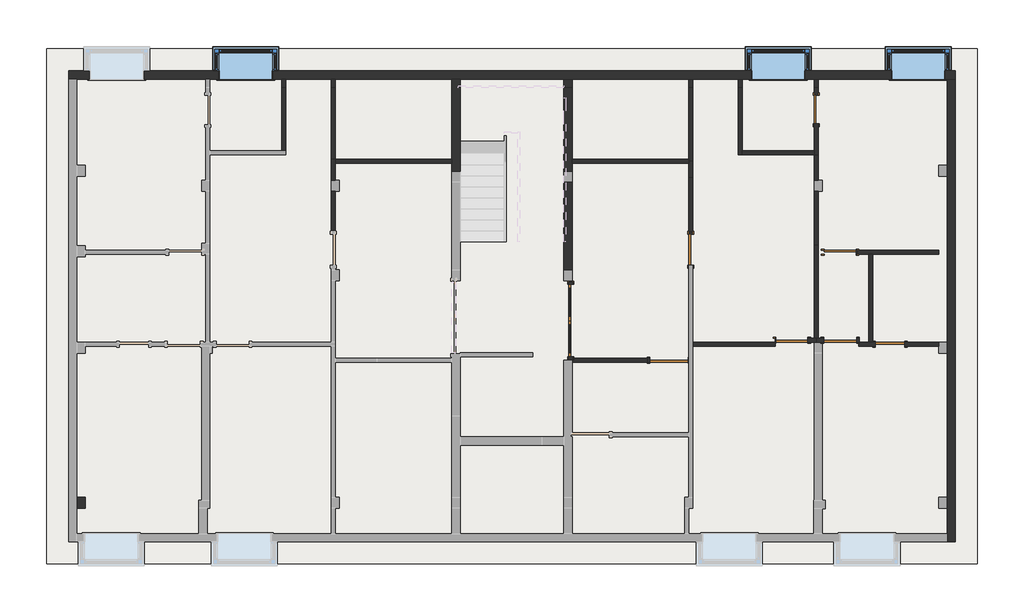
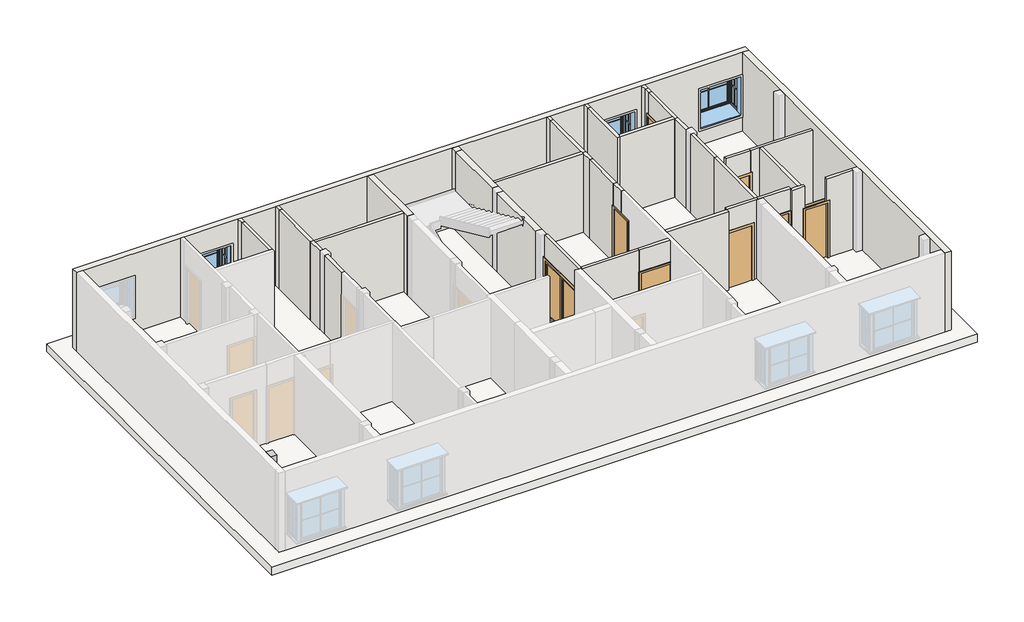
# One storey, part 2 of 3: 39 walls, 8 doors, 3 windows, 1 column, 1 slab.
"""IFC4 building model written with IfcOpenShell, lengths in millimetres."""

from ifc_helpers import new_model, si_unit, frame, origin, place, context, project, spatial, polyline, outline, extrude, faceted_brep, transform, mapped, element, save
from components import door_04ab2522, m_door_single_panel_05506f71, door_85b31ab1, door_1991e9a2, door_a431d384, door_82def9da, m_door_single_panel_3_x7_f8176753, window_19bbd869

model = new_model("IFC4")

# Units and contexts
model_context = context("Model", 3, world=origin())
ifc_project = project(units=[si_unit("LENGTHUNIT", "METRE", prefix="MILLI")], contexts=[model_context])

# Site, building, storey
site = spatial("IfcSite", under=ifc_project)
building = spatial("IfcBuilding", under=site)
storey = spatial("IfcBuildingStorey", under=building, Elevation=19202.4)

# Column
placement = place(None, origin())
element("IfcColumn", 1, ObjectType="Rectangular Column : 1'X 9\"", at=placement, inside=storey, context=model_context, shape_type="SweptSolid", body=[
    extrude(outline(polyline([(-12224.6987957, -3709.2932671), (-12224.6987957, -4014.0932671), (-12453.2987957, -4014.0932671), (-12453.2987957, -3709.2932671), (-12224.6987957, -3709.2932671)])), frame((0.0, 0.0, 19202.4), z_axis=(0.0, 0.0, 1.0), x_axis=(1.0, 0.0, 0.0)), (0.0, 0.0, 1.0), 3048.0),
])

# Doors
door_shape = door_04ab2522(model_context)
element("IfcDoor", 2, ObjectType="M_Door-Double-Glass : 6'7\"X7'", at=placement, inside=storey, context=model_context, shape_type="MappedRepresentation", body=[
    mapped(door_shape, transform((1217.5394962, 1183.3817656, 19202.4), x_axis=(0.0, 1.0, 0.0), y_axis=(-1.0, 0.0, 0.0), z_axis=(0.0, 0.0, 1.0))),
])
m_door_single_panel_shape = m_door_single_panel_05506f71(model_context)
element("IfcDoor", 3, ObjectType="M_Door-Single-Panel", at=placement, inside=storey, context=model_context, shape_type="MappedRepresentation", body=[
    mapped(m_door_single_panel_shape, transform((3933.4813133, 90.9578621, 19202.4), x_axis=(1.0, 0.0, 0.0), y_axis=(0.0, 1.0, 0.0), z_axis=(0.0, 0.0, 1.0))),
])
door_2_shape = door_85b31ab1(model_context)
element("IfcDoor", 4, ObjectType="M_Door-Single-Panel : 2'10\"X7' 2", at=placement, inside=storey, context=model_context, shape_type="MappedRepresentation", body=[
    mapped(door_2_shape, transform((4532.9512082, 3142.9626891, 19202.4), x_axis=(0.0, -1.0, 0.0), y_axis=(1.0, 0.0, 0.0), z_axis=(0.0, 0.0, 1.0))),
])
door_3_shape = door_1991e9a2(model_context)
element("IfcDoor", 5, ObjectType="M_Door-Single-Panel : 2'11\"X7' 3", at=placement, inside=storey, context=model_context, shape_type="MappedRepresentation", body=[
    mapped(door_3_shape, transform((7330.1405552, 640.4567334, 19202.4), x_axis=(1.0, 0.0, 0.0), y_axis=(0.0, 1.0, 0.0), z_axis=(0.0, 0.0, 1.0))),
])
element("IfcDoor", 6, ObjectType="M_Door-Single-Panel : 2'11\"X7' 3", at=placement, inside=storey, context=model_context, shape_type="MappedRepresentation", body=[
    mapped(door_3_shape, transform((8664.274939, 3078.8567332, 19202.4), x_axis=(-1.0, 0.0, 0.0), y_axis=(0.0, -1.0, 0.0), z_axis=(0.0, 0.0, 1.0))),
])
door_4_shape = door_a431d384(model_context)
element("IfcDoor", 7, ObjectType="M_Door-Single-Panel : 2'7\"X7' 2", at=placement, inside=storey, context=model_context, shape_type="MappedRepresentation", body=[
    mapped(door_4_shape, transform((8000.0512079, 7021.3751452, 19202.4), x_axis=(0.0, 1.0, 0.0), y_axis=(-1.0, 0.0, 0.0), z_axis=(0.0, 0.0, 1.0))),
])
door_5_shape = door_82def9da(model_context)
element("IfcDoor", 8, ObjectType="M_Door-Single-Panel : 2'8\"X7'", at=placement, inside=storey, context=model_context, shape_type="MappedRepresentation", body=[
    mapped(door_5_shape, transform((10046.0486694, 526.1567295, 19202.4), x_axis=(-1.0, 0.0, 0.0), y_axis=(0.0, -1.0, 0.0), z_axis=(0.0, 0.0, 1.0))),
])
m_door_single_panel_3_x7_shape = m_door_single_panel_3_x7_f8176753(model_context)
element("IfcDoor", 9, ObjectType="M_Door-Single-Panel : 3'X7'", at=placement, inside=storey, context=model_context, shape_type="MappedRepresentation", body=[
    mapped(m_door_single_panel_3_x7_shape, transform((8666.8012079, 640.4567334, 19202.4), x_axis=(-1.0, 0.0, 0.0), y_axis=(0.0, -1.0, 0.0), z_axis=(0.0, 0.0, 1.0))),
])

# Slab
element("IfcSlab", 10, ObjectType="Generic - 12\"", at=placement, inside=storey, context=model_context, shape_type="SweptSolid", body=[
    extrude(outline(polyline([(12464.1012075, 8698.6067329), (12464.1012075, -5550.7932662), (-13291.4987957, -5550.7932662), (-13291.4987957, 8698.6067329), (12464.1012075, 8698.6067329)])), frame((0.0, 0.0, 18897.6), z_axis=(0.0, 0.0, 1.0), x_axis=(1.0, 0.0, 0.0)), (0.0, 0.0, 1.0), 304.8),
])

# Walls
element("IfcWall", 11, ObjectType="4.5\"", at=placement, inside=storey, context=model_context, shape_type="SweptSolid", body=[
    extrude(outline(polyline([(3132.0737955, 22250.4), (3628.3344162, 22250.4), (3628.3344162, 19202.4), (3574.7626891, 19202.4), (3574.7626891, 21336.0), (3132.0737955, 21336.0), (3132.0737955, 22250.4)])), frame((4475.8012082, 0.0, 0.0), z_axis=(1.0, 0.0, 0.0), x_axis=(0.0, 1.0, 0.0)), (0.0, 0.0, 1.0), 114.3),
])
element("IfcWall", 12, ObjectType="4.5\"", at=placement, inside=storey, context=model_context, shape_type="Brep", body=[
    faceted_brep([(8000.0512079, 583.3067334, 19202.4), (8000.0512079, 583.3067334, 22250.4), (7942.9012047, 583.3067334, 22250.4), (6862.7668241, 583.3067334, 22250.4), (6862.7668241, 583.3067334, 19202.4), (6885.6405552, 583.3067334, 19202.4), (6885.6405552, 583.3067334, 21336.0), (7774.6405552, 583.3067334, 21336.0), (7774.6405552, 583.3067334, 19202.4), (7942.9012047, 583.3067334, 19202.4), (8000.0512079, 697.6067334, 22250.4), (8000.0512079, 697.6067334, 19202.4), (7942.9012079, 697.6067334, 19202.4), (7774.6405552, 697.6067334, 19202.4), (7774.6405552, 697.6067334, 21336.0), (6885.6405552, 697.6067334, 21336.0), (6885.6405552, 697.6067334, 19202.4), (6862.7668241, 697.6067334, 19202.4), (6862.7668241, 697.6067334, 22250.4), (7942.9012079, 697.6067334, 22250.4)], [[[0, 1, 2, 3, 4, 5, 6, 7, 8, 9]], [[10, 11, 12, 13, 14, 15, 16, 17, 18, 19]], [[4, 17, 16, 5]], [[11, 0, 9, 8, 13, 12]], [[1, 0, 11, 10]], [[3, 2, 1, 10, 19, 18]], [[4, 3, 18, 17]], [[7, 14, 13, 8]], [[14, 7, 6, 15]], [[15, 6, 5, 16]]]),
])
element("IfcWall", 13, ObjectType="4.5\"", at=placement, inside=storey, context=model_context, shape_type="Brep", body=[
    faceted_brep([(9187.5012047, 583.3067334, 19202.4), (9187.5012047, 583.3067334, 22250.4), (8171.5012047, 583.3067334, 22250.4), (8000.0512079, 583.3067334, 22250.4), (8000.0512079, 583.3067334, 19202.4), (8171.5012047, 583.3067334, 19202.4), (8209.6012079, 583.3067334, 19202.4), (8209.6012079, 583.3067334, 21336.0), (9124.0012079, 583.3067334, 21336.0), (9124.0012079, 583.3067334, 19202.4), (9187.5012047, 697.6067334, 22250.4), (9187.5012047, 697.6067334, 19202.4), (9124.0012079, 697.6067334, 19202.4), (9124.0012079, 697.6067334, 21336.0), (8209.6012079, 697.6067334, 21336.0), (8209.6012079, 697.6067334, 19202.4), (8057.2012079, 697.6067334, 19202.4), (8000.0512079, 697.6067334, 19202.4), (8000.0512079, 697.6067334, 22250.4), (8057.2012079, 697.6067334, 22250.4)], [[[0, 1, 2, 3, 4, 5, 6, 7, 8, 9]], [[10, 11, 12, 13, 14, 15, 16, 17, 18, 19]], [[11, 0, 9, 12]], [[4, 17, 16, 15, 6, 5]], [[1, 0, 11, 10]], [[3, 2, 1, 10, 19, 18]], [[4, 3, 18, 17]], [[7, 14, 13, 8]], [[8, 13, 12, 9]], [[14, 7, 6, 15]]]),
])
element("IfcWall", 14, ObjectType="4.5\"", at=placement, inside=storey, context=model_context, shape_type="SweptSolid", body=[
    extrude(outline(polyline([(19202.4, 9131.6486701), (22250.4, 9131.6486701), (22250.4, 8245.174939), (21336.0, 8245.174939), (21336.0, 9108.774939), (19202.4, 9108.774939), (19202.4, 9131.6486701)])), frame((0.0, 3021.7067332, 0.0), z_axis=(0.0, 1.0, 0.0), x_axis=(0.0, 0.0, 1.0)), (0.0, 0.0, 1.0), 114.3),
])
element("IfcWall", 15, ObjectType="4.5\"", at=placement, inside=storey, context=model_context, shape_type="Brep", body=[
    faceted_brep([(7942.9012079, 5764.9067329, 22250.4), (7942.9012079, 5879.2067329, 22250.4), (7942.9012079, 7415.0751452, 22250.4), (7942.9012079, 7415.0751452, 21336.0), (7942.9012079, 6627.6751452, 21336.0), (7942.9012079, 6627.6751452, 19202.4), (7942.9012079, 5879.2067329, 19202.4), (7942.9012079, 5764.9067329, 19202.4), (8057.2012079, 7415.0751452, 22250.4), (8057.2012079, 5764.9067329, 22250.4), (8057.2012079, 5764.9067329, 19202.4), (8057.2012079, 6627.6751452, 19202.4), (8057.2012079, 6627.6751452, 21336.0), (8057.2012079, 7415.0751452, 21336.0)], [[[0, 1, 2, 3, 4, 5, 6, 7]], [[8, 9, 10, 11, 12, 13]], [[10, 7, 6, 5, 11]], [[2, 1, 0, 9, 8]], [[2, 8, 13, 3]], [[12, 4, 3, 13]], [[4, 12, 11, 5]], [[0, 7, 10, 9]]]),
])
element("IfcWall", 16, ObjectType="4.5\"", at=placement, inside=storey, context=model_context, shape_type="SweptSolid", body=[
    extrude(outline(polyline([(21336.0, 4466.8813133), (19202.4, 4466.8813133), (19202.4, 4475.8012082), (22250.4, 4475.8012082), (22250.4, 3334.0114184), (19202.4, 3334.0114184), (19202.4, 3400.0813133), (21336.0, 3400.0813133), (21336.0, 4466.8813133)])), frame((0.0, 33.8078621, 0.0), z_axis=(0.0, 1.0, 0.0), x_axis=(0.0, 0.0, 1.0)), (0.0, 0.0, 1.0), 114.3),
])
element("IfcWall", 17, ObjectType="4.5\"", at=placement, inside=storey, context=model_context, shape_type="Brep", body=[
    faceted_brep([(1158.0082462, 2240.6567742, 19202.4), (1158.0082462, 2186.6817656, 19202.4), (1158.0082462, 2186.6817656, 21336.0), (1158.0082462, 180.0817656, 21336.0), (1158.0082462, 180.0817656, 19202.4), (1158.0082462, 90.9578621, 19202.4), (1158.0082462, 90.9578621, 22250.4), (1158.0082462, 2240.6567742, 22250.4), (1272.3082462, 2186.6817656, 21336.0), (1272.3082462, 2186.6817656, 19202.4), (1272.3082462, 2240.6567742, 19202.4), (1272.3082462, 2240.6567742, 22250.4), (1272.3082462, 148.1078621, 22250.4), (1272.3082462, 90.9578621, 22250.4), (1272.3082462, 90.9578621, 19202.4), (1272.3082462, 148.1078621, 19202.4), (1272.3082462, 180.0817656, 19202.4), (1272.3082462, 180.0817656, 21336.0), (1250.0012085, 90.9578621, 19202.4), (1250.0012085, 90.9578621, 22250.4)], [[[0, 1, 2, 3, 4, 5, 6, 7]], [[8, 9, 10, 11, 12, 13, 14, 15, 16, 17]], [[10, 9, 1, 0]], [[16, 15, 14, 18, 5, 4]], [[6, 5, 18, 14, 13, 19]], [[7, 6, 19, 13, 12, 11]], [[0, 7, 11, 10]], [[2, 1, 9, 8]], [[3, 2, 8, 17]], [[4, 3, 17, 16]]]),
])
element("IfcWall", 18, ObjectType="4.5\"", at=placement, inside=storey, context=model_context, shape_type="Brep", body=[
    faceted_brep([(1250.0012085, 5536.3067329, 19202.4), (4475.8012082, 5536.3067329, 19202.4), (4475.8012082, 5536.3067329, 22250.4), (1250.0012085, 5536.3067329, 22250.4), (1250.0012085, 5650.6067329, 19202.4), (1250.0012085, 5650.6067329, 22250.4), (4475.8012082, 5650.6067329, 22250.4), (4475.8012082, 5650.6067329, 19202.4), (4475.8012082, 5593.4567329, 19202.4), (4475.8012082, 5593.4567329, 22250.4)], [[[0, 1, 2, 3]], [[4, 5, 6, 7]], [[1, 0, 4, 7, 8]], [[3, 2, 9, 6, 5]], [[2, 1, 8, 7, 6, 9]], [[0, 3, 5, 4]]]),
])
element("IfcWall", 19, ObjectType="4.5\"", at=placement, inside=storey, context=model_context, shape_type="Brep", body=[
    faceted_brep([(7942.9012079, 7631.8067329, 19202.4), (7942.9012079, 7415.0751452, 19202.4), (7942.9012079, 7415.0751452, 21336.0), (7942.9012079, 7415.0751452, 22250.4), (7942.9012079, 7631.8067329, 22250.4), (8057.2012079, 7631.8067329, 19202.4), (8057.2012079, 7631.8067329, 22250.4), (8057.2012079, 7415.0751452, 22250.4), (8057.2012079, 7415.0751452, 21336.0), (8057.2012079, 7415.0751452, 19202.4)], [[[0, 1, 2, 3, 4]], [[5, 6, 7, 8, 9]], [[1, 0, 5, 9]], [[3, 2, 1, 9, 8, 7]], [[4, 3, 7, 6]], [[0, 4, 6, 5]]]),
])
element("IfcWall", 20, ObjectType="4.5\"", at=placement, inside=storey, context=model_context, shape_type="Brep", body=[
    faceted_brep([(8057.2012047, 3270.1432417, 19202.4), (8057.2012047, 4760.6824989, 19202.4), (8057.2012047, 4760.6824989, 22250.4), (8057.2012047, 3270.1432417, 22250.4), (7942.9012047, 3270.1432417, 19202.4), (7942.9012047, 3270.1432417, 22250.4), (7942.9012047, 4760.6824989, 22250.4), (7942.9012047, 4760.6824989, 19202.4), (7943.9040565, 4760.6824989, 19202.4), (7943.9040565, 4760.6824989, 22250.4)], [[[0, 1, 2, 3]], [[4, 5, 6, 7]], [[1, 0, 4, 7, 8]], [[2, 1, 8, 7, 6, 9]], [[3, 2, 9, 6, 5]], [[0, 3, 5, 4]]]),
])
element("IfcWall", 21, ObjectType="4.5\"", at=placement, inside=storey, context=model_context, shape_type="Brep", body=[
    faceted_brep([(7942.9012079, 3270.1432417, 19202.4), (7942.9012079, 697.6067334, 19202.4), (7942.9012079, 697.6067334, 22250.4), (7942.9012079, 3270.1432417, 22250.4), (8057.2012079, 3270.1432417, 19202.4), (8057.2012079, 3270.1432417, 22250.4), (8057.2012079, 697.6067334, 22250.4), (8057.2012079, 697.6067334, 19202.4), (8000.0512079, 697.6067334, 19202.4), (8000.0512079, 697.6067334, 22250.4)], [[[0, 1, 2, 3]], [[4, 5, 6, 7]], [[1, 0, 4, 7, 8]], [[3, 2, 9, 6, 5]], [[0, 3, 5, 4]], [[2, 1, 8, 7, 6, 9]]]),
])
element("IfcWall", 22, ObjectType="4.5\"", at=placement, inside=storey, context=model_context, shape_type="SweptSolid", body=[
    extrude(outline(polyline([(8058.2040565, 5763.9824989), (8058.2040565, 5065.4824989), (7943.9040565, 5065.4824989), (7943.9040565, 5763.9824989), (8058.2040565, 5763.9824989)])), frame((0.0, 0.0, 19202.4), z_axis=(0.0, 0.0, 1.0), x_axis=(1.0, 0.0, 0.0)), (0.0, 0.0, 1.0), 3048.0),
])
element("IfcWall", 23, ObjectType="4.5\"", at=placement, inside=storey, context=model_context, shape_type="SweptSolid", body=[
    extrude(outline(polyline([(5961.701208, 7860.4067329), (5961.701208, 7631.8067329), (5847.401208, 7631.8067329), (5847.401208, 7860.4067329), (5961.701208, 7860.4067329)])), frame((0.0, 0.0, 19202.4), z_axis=(0.0, 0.0, 1.0), x_axis=(1.0, 0.0, 0.0)), (0.0, 0.0, 1.0), 3048.0),
])
element("IfcWall", 24, ObjectType="4.5\"", at=placement, inside=storey, context=model_context, shape_type="SweptSolid", body=[
    extrude(outline(polyline([(8057.2012079, 7860.4067329), (8057.2012079, 7631.8067329), (7942.9012079, 7631.8067329), (7942.9012079, 7860.4067329), (8057.2012079, 7860.4067329)])), frame((0.0, 0.0, 19202.4), z_axis=(0.0, 0.0, 1.0), x_axis=(1.0, 0.0, 0.0)), (0.0, 0.0, 1.0), 3048.0),
])
element("IfcWall", 25, ObjectType="4.5\"", at=placement, inside=storey, context=model_context, shape_type="SweptSolid", body=[
    extrude(outline(polyline([(4590.1012082, 7860.4067329), (4590.1012082, 7631.8067329), (4475.8012082, 7631.8067329), (4475.8012082, 7860.4067329), (4590.1012082, 7860.4067329)])), frame((0.0, 0.0, 19202.4), z_axis=(0.0, 0.0, 1.0), x_axis=(1.0, 0.0, 0.0)), (0.0, 0.0, 1.0), 3048.0),
])
element("IfcWall", 26, ObjectType="4.5\"", at=placement, inside=storey, context=model_context, shape_type="SweptSolid", body=[
    extrude(outline(polyline([(-6674.7987994, 7860.4067329), (-6674.7987994, 7631.8067329), (-6789.0987994, 7631.8067329), (-6789.0987994, 7860.4067329), (-6674.7987994, 7860.4067329)])), frame((0.0, 0.0, 19202.4), z_axis=(0.0, 0.0, 1.0), x_axis=(1.0, 0.0, 0.0)), (0.0, 0.0, 1.0), 3048.0),
])
element("IfcWall", 27, ObjectType="4.5\"", at=placement, inside=storey, context=model_context, shape_type="SweptSolid", body=[
    extrude(outline(polyline([(-5303.1987995, 7860.4067329), (-5303.1987995, 7631.8067329), (-5417.4987995, 7631.8067329), (-5417.4987995, 7860.4067329), (-5303.1987995, 7860.4067329)])), frame((0.0, 0.0, 19202.4), z_axis=(0.0, 0.0, 1.0), x_axis=(1.0, 0.0, 0.0)), (0.0, 0.0, 1.0), 3048.0),
])
element("IfcWall", 28, ObjectType="4.5\"", at=placement, inside=storey, context=model_context, shape_type="SweptSolid", body=[
    extrude(outline(polyline([(1272.3082462, 148.1078621), (3334.0114184, 148.1078621), (3334.0114184, 33.8078621), (1250.0012085, 33.8078621), (1250.0012085, 90.9578621), (1272.3082462, 90.9578621), (1272.3082462, 148.1078621)])), frame((0.0, 0.0, 19202.4), z_axis=(0.0, 0.0, 1.0), x_axis=(1.0, 0.0, 0.0)), (0.0, 0.0, 1.0), 3048.0),
])
element("IfcWall", 29, ObjectType="4.5\" 2", at=placement, inside=storey, context=model_context, shape_type="SweptSolid", body=[
    extrude(outline(polyline([(-6674.7987994, 7631.8067329), (-6674.7987994, 5879.2067329), (-6789.0987994, 5879.2067329), (-6789.0987994, 7631.8067329), (-6674.7987994, 7631.8067329)])), frame((0.0, 0.0, 19202.4), z_axis=(0.0, 0.0, 1.0), x_axis=(1.0, 0.0, 0.0)), (0.0, 0.0, 1.0), 3048.0),
])
element("IfcWall", 30, ObjectType="4.5\" 2", at=placement, inside=storey, context=model_context, shape_type="SweptSolid", body=[
    extrude(outline(polyline([(-5303.1987995, 4761.606733), (-5303.1987995, 3671.8272228), (-5417.4987995, 3671.8272228), (-5417.4987995, 4761.606733), (-5303.1987995, 4761.606733)])), frame((0.0, 0.0, 19202.4), z_axis=(0.0, 0.0, 1.0), x_axis=(1.0, 0.0, 0.0)), (0.0, 0.0, 1.0), 3048.0),
])
element("IfcWall", 31, ObjectType="4.5\" 2", at=placement, inside=storey, context=model_context, shape_type="Brep", body=[
    faceted_brep([(-5303.1987995, 5066.406733, 19202.4), (-5303.1987995, 5536.3067329, 19202.4), (-5303.1987995, 5650.6067329, 19202.4), (-5303.1987995, 5650.6067329, 22250.4), (-5303.1987995, 5536.3067329, 22250.4), (-5303.1987995, 5066.406733, 22250.4), (-5417.4987995, 5066.406733, 19202.4), (-5417.4987995, 5066.406733, 22250.4), (-5417.4987995, 5650.6067329, 22250.4), (-5417.4987995, 5650.6067329, 19202.4)], [[[0, 1, 2, 3, 4, 5]], [[6, 7, 8, 9]], [[2, 1, 0, 6, 9]], [[5, 4, 3, 8, 7]], [[0, 5, 7, 6]], [[3, 2, 9, 8]]]),
])
element("IfcWall", 32, ObjectType="4.5\" 2", at=placement, inside=storey, context=model_context, shape_type="SweptSolid", body=[
    extrude(outline(polyline([(-2077.3987998, 5536.3067329), (-5303.1987995, 5536.3067329), (-5303.1987995, 5650.6067329), (-2077.3987998, 5650.6067329), (-2077.3987998, 5536.3067329)])), frame((0.0, 0.0, 19202.4), z_axis=(0.0, 0.0, 1.0), x_axis=(1.0, 0.0, 0.0)), (0.0, 0.0, 1.0), 3048.0),
])
element("IfcWall", 33, ObjectType="4.5\" 2", at=placement, inside=storey, context=model_context, shape_type="SweptSolid", body=[
    extrude(outline(polyline([(-5417.4987995, 5650.6067329), (-5417.4987995, 7631.8067329), (-5303.1987995, 7631.8067329), (-5303.1987995, 5650.6067329), (-5417.4987995, 5650.6067329)])), frame((0.0, 0.0, 19202.4), z_axis=(0.0, 0.0, 1.0), x_axis=(1.0, 0.0, 0.0)), (0.0, 0.0, 1.0), 3048.0),
])
element("IfcWall", 34, ObjectType="4.5\" 2", at=placement, inside=storey, context=model_context, shape_type="Brep", body=[
    faceted_brep([(4475.8012082, 5593.4567329, 19202.4), (4475.8012082, 5536.3067329, 19202.4), (4475.8012082, 5136.6567004, 19202.4), (4475.8012082, 5136.6567004, 22250.4), (4475.8012082, 5536.3067329, 22250.4), (4475.8012082, 5593.4567329, 22250.4), (4590.1012082, 5593.4567329, 19202.4), (4590.1012082, 5593.4567329, 22250.4), (4590.1012082, 5136.6567004, 22250.4), (4590.1012082, 5136.6567004, 19202.4)], [[[0, 1, 2, 3, 4, 5]], [[6, 7, 8, 9]], [[2, 1, 0, 6, 9]], [[3, 2, 9, 8]], [[5, 4, 3, 8, 7]], [[0, 5, 7, 6]]]),
])
element("IfcWall", 35, ObjectType="4.5\" 2", at=placement, inside=storey, context=model_context, shape_type="SweptSolid", body=[
    extrude(outline(polyline([(4475.8012082, 3628.3344162), (4475.8012082, 5136.6567004), (4590.1012082, 5136.6567004), (4590.1012082, 3628.3344162), (4475.8012082, 3628.3344162)])), frame((0.0, 0.0, 19202.4), z_axis=(0.0, 0.0, 1.0), x_axis=(1.0, 0.0, 0.0)), (0.0, 0.0, 1.0), 3048.0),
])
element("IfcWall", 36, ObjectType="4.5\" 2", at=placement, inside=storey, context=model_context, shape_type="SweptSolid", body=[
    extrude(outline(polyline([(6862.7668241, 469.0067334), (4590.1012082, 469.0067334), (4590.1012082, 583.3067334), (6862.7668241, 583.3067334), (6862.7668241, 469.0067334)])), frame((0.0, 0.0, 19202.4), z_axis=(0.0, 0.0, 1.0), x_axis=(1.0, 0.0, 0.0)), (0.0, 0.0, 1.0), 3048.0),
])
element("IfcWall", 37, ObjectType="4.5\" 2", at=placement, inside=storey, context=model_context, shape_type="Brep", body=[
    faceted_brep([(9182.4486694, 469.0067295, 19202.4), (9639.6486694, 469.0067295, 19202.4), (9639.6486694, 469.0067295, 22250.4), (9182.4486694, 469.0067295, 22250.4), (9182.4486694, 583.3067295, 19202.4), (9182.4486694, 583.3067295, 22250.4), (9451.1098918, 583.3067295, 22250.4), (9565.4098918, 583.3067295, 22250.4), (9639.6486694, 583.3067295, 22250.4), (9639.6486694, 583.3067295, 19202.4), (9565.4098918, 583.3067295, 19202.4), (9451.1098918, 583.3067295, 19202.4)], [[[0, 1, 2, 3]], [[4, 5, 6, 7, 8, 9, 10, 11]], [[1, 0, 4, 11, 10, 9]], [[2, 1, 9, 8]], [[3, 2, 8, 7, 6, 5]], [[0, 3, 5, 4]]]),
])
element("IfcWall", 38, ObjectType="4.5\" 2", at=placement, inside=storey, context=model_context, shape_type="SweptSolid", body=[
    extrude(outline(polyline([(19202.4, 11397.3012075), (22250.4, 11397.3012075), (22250.4, 10443.8236977), (21336.0, 10443.8236977), (21336.0, 10452.4486694), (19202.4, 10452.4486694), (19202.4, 11397.3012075)])), frame((0.0, 469.0067295, 0.0), z_axis=(0.0, 1.0, 0.0), x_axis=(0.0, 0.0, 1.0)), (0.0, 0.0, 1.0), 114.3),
])
element("IfcWall", 39, ObjectType="4.5\" 2", at=placement, inside=storey, context=model_context, shape_type="SweptSolid", body=[
    extrude(outline(polyline([(9565.4098918, 3021.7067332), (9565.4098918, 583.3067295), (9451.1098918, 583.3067295), (9451.1098918, 3021.7067332), (9565.4098918, 3021.7067332)])), frame((0.0, 0.0, 19202.4), z_axis=(0.0, 0.0, 1.0), x_axis=(1.0, 0.0, 0.0)), (0.0, 0.0, 1.0), 3048.0),
])
element("IfcWall", 40, ObjectType="4.5\" 2", at=placement, inside=storey, context=model_context, shape_type="Brep", body=[
    faceted_brep([(9131.6486701, 3021.7067332, 19202.4), (9451.1098918, 3021.7067332, 19202.4), (9565.4098918, 3021.7067332, 19202.4), (11397.3012075, 3021.7067332, 19202.4), (11397.3012075, 3021.7067332, 22250.4), (9565.4098918, 3021.7067332, 22250.4), (9451.1098918, 3021.7067332, 22250.4), (9131.6486701, 3021.7067332, 22250.4), (9131.6486701, 3136.0067332, 19202.4), (9131.6486701, 3136.0067332, 22250.4), (11397.3012075, 3136.0067332, 22250.4), (11397.3012075, 3136.0067332, 19202.4)], [[[0, 1, 2, 3, 4, 5, 6, 7]], [[8, 9, 10, 11]], [[3, 2, 1, 0, 8, 11]], [[4, 3, 11, 10]], [[7, 6, 5, 4, 10, 9]], [[0, 7, 9, 8]]]),
])
element("IfcWall", 41, ObjectType="4.5\" 2", at=placement, inside=storey, context=model_context, shape_type="Brep", body=[
    faceted_brep([(4590.1012082, 5593.4567329, 19202.4), (4590.1012082, 7631.8067329, 19202.4), (4590.1012082, 7631.8067329, 22250.4), (4590.1012082, 5593.4567329, 22250.4), (4475.8012082, 5593.4567329, 19202.4), (4475.8012082, 5593.4567329, 22250.4), (4475.8012082, 5650.6067329, 22250.4), (4475.8012082, 7631.8067329, 22250.4), (4475.8012082, 7631.8067329, 19202.4), (4475.8012082, 5650.6067329, 19202.4)], [[[0, 1, 2, 3]], [[4, 5, 6, 7, 8, 9]], [[1, 0, 4, 9, 8]], [[2, 1, 8, 7]], [[3, 2, 7, 6, 5]], [[0, 3, 5, 4]]]),
])
element("IfcWall", 42, ObjectType="4.5\" 2", at=placement, inside=storey, context=model_context, shape_type="Brep", body=[
    faceted_brep([(5847.401208, 7631.8067329, 19202.4), (5847.401208, 5764.9067329, 19202.4), (5847.401208, 5764.9067329, 22250.4), (5847.401208, 7631.8067329, 22250.4), (5961.701208, 7631.8067329, 19202.4), (5961.701208, 7631.8067329, 22250.4), (5961.701208, 5879.2067329, 22250.4), (5961.701208, 5764.9067329, 22250.4), (5961.701208, 5764.9067329, 19202.4), (5961.701208, 5879.2067329, 19202.4)], [[[0, 1, 2, 3]], [[4, 5, 6, 7, 8, 9]], [[1, 0, 4, 9, 8]], [[3, 2, 7, 6, 5]], [[0, 3, 5, 4]], [[2, 1, 8, 7]]]),
])
element("IfcWall", 43, ObjectType="4.5\" 2", at=placement, inside=storey, context=model_context, shape_type="SweptSolid", body=[
    extrude(outline(polyline([(7942.9012079, 5764.9067329), (5961.701208, 5764.9067329), (5961.701208, 5879.2067329), (7942.9012079, 5879.2067329), (7942.9012079, 5764.9067329)])), frame((0.0, 0.0, 19202.4), z_axis=(0.0, 0.0, 1.0), x_axis=(1.0, 0.0, 0.0)), (0.0, 0.0, 1.0), 3048.0),
])
element("IfcWall", 44, ObjectType="9\"", at=placement, inside=storey, context=model_context, shape_type="Brep", body=[
    faceted_brep([(-12681.8987957, 7860.4067329, 19202.4), (-12453.2987957, 7860.4067329, 19202.4), (-8884.5987992, 7860.4067329, 19202.4), (-8770.2987992, 7860.4067329, 19202.4), (-6789.0987994, 7860.4067329, 19202.4), (-6674.7987994, 7860.4067329, 19202.4), (-5417.4987995, 7860.4067329, 19202.4), (-5303.1987995, 7860.4067329, 19202.4), (-2074.1417538, 7860.4067329, 19202.4), (-1845.5417538, 7860.4067329, 19202.4), (1021.4012085, 7860.4067329, 19202.4), (1250.0012085, 7860.4067329, 19202.4), (4475.8012082, 7860.4067329, 19202.4), (4590.1012082, 7860.4067329, 19202.4), (5847.401208, 7860.4067329, 19202.4), (5961.701208, 7860.4067329, 19202.4), (7942.9012079, 7860.4067329, 19202.4), (8057.2012079, 7860.4067329, 19202.4), (11625.9012075, 7860.4067329, 19202.4), (11854.5012075, 7860.4067329, 19202.4), (11854.5012075, 7860.4067329, 22250.4), (11625.9012075, 7860.4067329, 22250.4), (8057.2012079, 7860.4067329, 22250.4), (7942.9012079, 7860.4067329, 22250.4), (5961.701208, 7860.4067329, 22250.4), (5847.401208, 7860.4067329, 22250.4), (4590.1012082, 7860.4067329, 22250.4), (4475.8012082, 7860.4067329, 22250.4), (1250.0012085, 7860.4067329, 22250.4), (1021.4012085, 7860.4067329, 22250.4), (-1845.5417538, 7860.4067329, 22250.4), (-2074.1417538, 7860.4067329, 22250.4), (-5303.1987995, 7860.4067329, 22250.4), (-5417.4987995, 7860.4067329, 22250.4), (-6674.7987994, 7860.4067329, 22250.4), (-6789.0987994, 7860.4067329, 22250.4), (-8770.2987992, 7860.4067329, 22250.4), (-8884.5987992, 7860.4067329, 22250.4), (-12453.2987957, 7860.4067329, 22250.4), (-12681.8987957, 7860.4067329, 22250.4), (11575.8012075, 7860.4067329, 21353.2), (11575.8012075, 7860.4067329, 19802.4), (10075.8012075, 7860.4067329, 19802.4), (10075.8012075, 7860.4067329, 21353.2), (7702.301208, 7860.4067329, 21353.2), (7702.301208, 7860.4067329, 19802.4), (6202.301208, 7860.4067329, 19802.4), (6202.301208, 7860.4067329, 21353.2), (-7029.6987993, 7860.4067329, 21353.2), (-7029.6987993, 7860.4067329, 19802.4), (-8529.6987993, 7860.4067329, 19802.4), (-8529.6987993, 7860.4067329, 21353.2), (-10598.3987957, 7860.4067329, 21353.2), (-10598.3987957, 7860.4067329, 19802.4), (-12098.3987957, 7860.4067329, 19802.4), (-12098.3987957, 7860.4067329, 21353.2), (-12681.8987957, 8089.0067329, 19202.4), (-12681.8987957, 8089.0067329, 22250.4), (11854.5012075, 8089.0067329, 22250.4), (11854.5012075, 8089.0067329, 19202.4), (11575.8012075, 8089.0067329, 21353.2), (10075.8012075, 8089.0067329, 21353.2), (10075.8012075, 8089.0067329, 19802.4), (11575.8012075, 8089.0067329, 19802.4), (7702.301208, 8089.0067329, 21353.2), (6202.301208, 8089.0067329, 21353.2), (6202.301208, 8089.0067329, 19802.4), (7702.301208, 8089.0067329, 19802.4), (-7029.6987993, 8089.0067329, 21353.2), (-8529.6987993, 8089.0067329, 21353.2), (-8529.6987993, 8089.0067329, 19802.4), (-7029.6987993, 8089.0067329, 19802.4), (-10598.3987957, 8089.0067329, 21353.2), (-12098.3987957, 8089.0067329, 21353.2), (-12098.3987957, 8089.0067329, 19802.4), (-10598.3987957, 8089.0067329, 19802.4)], [[[0, 1, 2, 3, 4, 5, 6, 7, 8, 9, 10, 11, 12, 13, 14, 15, 16, 17, 18, 19, 20, 21, 22, 23, 24, 25, 26, 27, 28, 29, 30, 31, 32, 33, 34, 35, 36, 37, 38, 39], [40, 41, 42, 43], [44, 45, 46, 47], [48, 49, 50, 51], [52, 53, 54, 55]], [[56, 57, 58, 59], [60, 61, 62, 63], [64, 65, 66, 67], [68, 69, 70, 71], [72, 73, 74, 75]], [[19, 18, 17, 16, 15, 14, 13, 12, 11, 10, 9, 8, 7, 6, 5, 4, 3, 2, 1, 0, 56, 59]], [[39, 38, 37, 36, 35, 34, 33, 32, 31, 30, 29, 28, 27, 26, 25, 24, 23, 22, 21, 20, 58, 57]], [[20, 19, 59, 58]], [[0, 39, 57, 56]], [[41, 40, 60, 63]], [[42, 41, 63, 62]], [[43, 42, 62, 61]], [[40, 43, 61, 60]], [[45, 44, 64, 67]], [[46, 45, 67, 66]], [[47, 46, 66, 65]], [[44, 47, 65, 64]], [[49, 48, 68, 71]], [[50, 49, 71, 70]], [[51, 50, 70, 69]], [[48, 51, 69, 68]], [[53, 52, 72, 75]], [[54, 53, 75, 74]], [[55, 54, 74, 73]], [[52, 55, 73, 72]]]),
])
element("IfcWall", 45, ObjectType="9\"", at=placement, inside=storey, context=model_context, shape_type="Brep", body=[
    faceted_brep([(11625.9012075, 7860.4067329, 19202.4), (11625.9012075, 5479.1567329, 19202.4), (11625.9012075, 5174.3567329, 19202.4), (11625.9012075, 583.3067295, 19202.4), (11625.9012075, 278.5067295, 19202.4), (11625.9012075, -3709.2932671, 19202.4), (11625.9012075, -4014.0932671, 19202.4), (11625.9012075, -4712.5932662, 19202.4), (11625.9012075, -4941.1932662, 19202.4), (11625.9012075, -4941.1932662, 22250.4), (11625.9012075, -4712.5932662, 22250.4), (11625.9012075, -4014.0932671, 22250.4), (11625.9012075, -3709.2932671, 22250.4), (11625.9012075, 278.5067295, 22250.4), (11625.9012075, 583.3067295, 22250.4), (11625.9012075, 5174.3567329, 22250.4), (11625.9012075, 5479.1567329, 22250.4), (11625.9012075, 7860.4067329, 22250.4), (11854.5012075, 7860.4067329, 19202.4), (11854.5012075, 7860.4067329, 22250.4), (11854.5012075, -4941.1932662, 22250.4), (11854.5012075, -4941.1932662, 19202.4)], [[[0, 1, 2, 3, 4, 5, 6, 7, 8, 9, 10, 11, 12, 13, 14, 15, 16, 17]], [[18, 19, 20, 21]], [[8, 7, 6, 5, 4, 3, 2, 1, 0, 18, 21]], [[17, 16, 15, 14, 13, 12, 11, 10, 9, 20, 19]], [[0, 17, 19, 18]], [[9, 8, 21, 20]]]),
])
element("IfcWall", 46, ObjectType="9\"", at=placement, inside=storey, context=model_context, shape_type="SweptSolid", body=[
    extrude(outline(polyline([(-2074.1417538, 5320.4067329), (-2074.1417538, 7860.4067329), (-1845.5417538, 7860.4067329), (-1845.5417538, 5320.4067329), (-2074.1417538, 5320.4067329)])), frame((0.0, 0.0, 19202.4), z_axis=(0.0, 0.0, 1.0), x_axis=(1.0, 0.0, 0.0)), (0.0, 0.0, 1.0), 3048.0),
])
element("IfcWall", 47, ObjectType="9\"", at=placement, inside=storey, context=model_context, shape_type="Brep", body=[
    faceted_brep([(1021.4012085, 7631.8067329, 19202.4), (1021.4012085, 5320.4067329, 19202.4), (1021.4012085, 5320.4067329, 22250.4), (1021.4012085, 7631.8067329, 22250.4), (1250.0012085, 7631.8067329, 19202.4), (1250.0012085, 7631.8067329, 22250.4), (1250.0012085, 5650.6067329, 22250.4), (1250.0012085, 5536.3067329, 22250.4), (1250.0012085, 5320.4067329, 22250.4), (1250.0012085, 5320.4067329, 19202.4), (1250.0012085, 5536.3067329, 19202.4), (1250.0012085, 5650.6067329, 19202.4)], [[[0, 1, 2, 3]], [[4, 5, 6, 7, 8, 9, 10, 11]], [[1, 0, 4, 11, 10, 9]], [[2, 1, 9, 8]], [[3, 2, 8, 7, 6, 5]], [[0, 3, 5, 4]]]),
])
element("IfcWall", 48, ObjectType="9\"", at=placement, inside=storey, context=model_context, shape_type="Brep", body=[
    faceted_brep([(1021.4012085, 5015.6067329, 19202.4), (1021.4012085, 2589.9067742, 19202.4), (1021.4012085, 2589.9067742, 22250.4), (1021.4012085, 5015.6067329, 22250.4), (1250.0012085, 5015.6067329, 19202.4), (1250.0012085, 5015.6067329, 22250.4), (1250.0012085, 2589.9067742, 22250.4), (1250.0012085, 2589.9067742, 19202.4), (1024.6582462, 2589.9067742, 19202.4), (1024.6582462, 2589.9067742, 22250.4)], [[[0, 1, 2, 3]], [[4, 5, 6, 7]], [[1, 0, 4, 7, 8]], [[2, 1, 8, 7, 6, 9]], [[3, 2, 9, 6, 5]], [[0, 3, 5, 4]]]),
])
element("IfcWall", 49, ObjectType="9\"", at=placement, inside=storey, context=model_context, shape_type="SweptSolid", body=[
    extrude(outline(polyline([(1250.0012085, 7860.4067329), (1250.0012085, 7631.8067329), (1021.4012085, 7631.8067329), (1021.4012085, 7860.4067329), (1250.0012085, 7860.4067329)])), frame((0.0, 0.0, 19202.4), z_axis=(0.0, 0.0, 1.0), x_axis=(1.0, 0.0, 0.0)), (0.0, 0.0, 1.0), 3048.0),
])

# Windows
window_shape = window_19bbd869(model_context)
element("IfcWindow", 50, ObjectType="4'.8\"x3'.8\"", at=placement, inside=storey, context=model_context, shape_type="MappedRepresentation", body=[
    mapped(window_shape, transform((-7779.6987993, 7974.7067329, 19202.4), x_axis=(1.0, 0.0, 0.0), y_axis=(0.0, 1.0, 0.0), z_axis=(0.0, 0.0, 1.0))),
])
element("IfcWindow", 51, ObjectType="4'.8\"x3'.8\"", at=placement, inside=storey, context=model_context, shape_type="MappedRepresentation", body=[
    mapped(window_shape, transform((6952.301208, 7974.7067329, 19202.4), x_axis=(1.0, 0.0, 0.0), y_axis=(0.0, 1.0, 0.0), z_axis=(0.0, 0.0, 1.0))),
])
element("IfcWindow", 52, ObjectType="4'.8\"x3'.8\"", at=placement, inside=storey, context=model_context, shape_type="MappedRepresentation", body=[
    mapped(window_shape, transform((10825.8012075, 7974.7067329, 19202.4), x_axis=(1.0, 0.0, 0.0), y_axis=(0.0, 1.0, 0.0), z_axis=(0.0, 0.0, 1.0))),
])

save(model, "model.ifc")

# Revit data of these elements
# Type "Rectangular Column : 1'X 9\""
#   Assembly Code = "B1010200"
#   Depth = 1' - 0"
#   Offset Base = 0' - 0"
#   Offset Top = 0' - 0"
#   Width = 0' - 9"
#   Material = none
# Type "M_Door-Double-Glass : 6'7\"X7'"
#   Type Mark = "16"
#   Construction Type Id = "opn-d45"
#   Assembly Code = "C1020"
#   Analytic Construction = "Wood frame, double glass door "
#   W = 3' - 3 1/2"
#   Thickness = 0' - 1.9685"
#   Thermal Resistance (R) = 1.8150 (h·ft²·°F)/BTU
#   Swing Angle [instance default] = 90.00°
#   Heat Transfer Coefficient (U) = 0.5510 BTU/(h·ft²·°F)
#   Height = 7' - 0"
#   Bottom Rail = 0' - 3.93701"
#   Top Rail = 0' - 3.93701"
#   Stiles = 0' - 3.93701"
#   Trim Projection = 0' - 0.98425"
#   Trim Width = 0' - 3.14961"
#   Width = 6' - 7"
#   Define Thermal Properties by = 1
#   Glazing = Glass
#   Panel Material = Wood - Birch - Solid Stained Light Low Gloss
#   Trim Material = Paint - Sienna
#   Visual Light Transmittance = 0
#   Solar Heat Gain Coefficient = 0
#   Function = (empty or 0)
#   Wall Closure = (empty or 0)
# Type "M_Door-Single-Panel"
#   Type Mark = "14"
#   Construction Type Id = "DOOR"
#   Assembly Code = "C1020300"
#   Analytic Construction = "Wooden"
#   Thickness = 0' - 1.9685"
#   Thermal Resistance (R) = 2.5876 (h·ft²·°F)/BTU
#   Swing Angle [instance default] = 90.00°
#   Heat Transfer Coefficient (U) = 0.3865 BTU/(h·ft²·°F)
#   Height = 7' - 0"
#   Trim Projection Ext = 0' - 0.98425"
#   Trim Projection Int = 0' - 0.98425"
#   Trim Width = 0' - 3.14961"
#   Width = 3' - 6"
#   Define Thermal Properties by = 1
#   Panel Material = Wood - Birch - Solid Stained Light Low Gloss
#   Trim Material = Paint - Sienna
#   Visual Light Transmittance = 0
#   Solar Heat Gain Coefficient = 0
#   Function = (empty or 0)
#   Wall Closure = (empty or 0)
# Type "M_Door-Single-Panel : 2'10\"X7' 2"
#   Type Mark = "10"
#   Construction Type Id = "DOOR"
#   Assembly Code = "C1020300"
#   Analytic Construction = "Wooden"
#   Thickness = 0' - 1.9685"
#   Thermal Resistance (R) = 2.5876 (h·ft²·°F)/BTU
#   Swing Angle [instance default] = 90.00°
#   Heat Transfer Coefficient (U) = 0.3865 BTU/(h·ft²·°F)
#   Height = 7' - 0"
#   Trim Projection Ext = 0' - 0.98425"
#   Trim Projection Int = 0' - 0.98425"
#   Trim Width = 0' - 3.14961"
#   Width = 2' - 10"
#   Define Thermal Properties by = 1
#   Panel Material = Wood - Birch - Solid Stained Light Low Gloss
#   Trim Material = Paint - Sienna
#   Visual Light Transmittance = 0
#   Solar Heat Gain Coefficient = 0
#   Function = (empty or 0)
#   Wall Closure = (empty or 0)
# Type "M_Door-Single-Panel : 2'11\"X7' 3"
#   Type Mark = "12"
#   Construction Type Id = "DOOR"
#   Assembly Code = "C1020300"
#   Analytic Construction = "Wooden"
#   Thickness = 0' - 1.9685"
#   Thermal Resistance (R) = 2.5876 (h·ft²·°F)/BTU
#   Swing Angle [instance default] = 90.00°
#   Heat Transfer Coefficient (U) = 0.3865 BTU/(h·ft²·°F)
#   Height = 7' - 0"
#   Trim Projection Ext = 0' - 0.98425"
#   Trim Projection Int = 0' - 0.98425"
#   Trim Width = 0' - 3.14961"
#   Width = 2' - 11"
#   Define Thermal Properties by = 1
#   Panel Material = Wood - Birch - Solid Stained Light Low Gloss
#   Trim Material = Paint - Sienna
#   Visual Light Transmittance = 0
#   Solar Heat Gain Coefficient = 0
#   Function = (empty or 0)
#   Wall Closure = (empty or 0)
# Type "M_Door-Single-Panel : 2'7\"X7' 2"
#   Type Mark = "13"
#   Construction Type Id = "DOOR"
#   Assembly Code = "C1020300"
#   Analytic Construction = "Wooden"
#   Thickness = 0' - 1.9685"
#   Thermal Resistance (R) = 2.5876 (h·ft²·°F)/BTU
#   Swing Angle [instance default] = 90.00°
#   Heat Transfer Coefficient (U) = 0.3865 BTU/(h·ft²·°F)
#   Height = 7' - 0"
#   Trim Projection Ext = 0' - 0.98425"
#   Trim Projection Int = 0' - 0.98425"
#   Trim Width = 0' - 3.14961"
#   Width = 2' - 7"
#   Define Thermal Properties by = 1
#   Panel Material = Wood - Birch - Solid Stained Light Low Gloss
#   Trim Material = Paint - Sienna
#   Visual Light Transmittance = 0
#   Solar Heat Gain Coefficient = 0
#   Function = (empty or 0)
#   Wall Closure = (empty or 0)
# Type "M_Door-Single-Panel : 2'8\"X7'"
#   Type Mark = "9"
#   Construction Type Id = "DOOR"
#   Assembly Code = "C1020300"
#   Analytic Construction = "Wooden"
#   Thickness = 0' - 1.9685"
#   Thermal Resistance (R) = 2.5876 (h·ft²·°F)/BTU
#   Swing Angle [instance default] = 90.00°
#   Heat Transfer Coefficient (U) = 0.3865 BTU/(h·ft²·°F)
#   Height = 7' - 0"
#   Trim Projection Ext = 0' - 0.98425"
#   Trim Projection Int = 0' - 0.98425"
#   Trim Width = 0' - 3.14961"
#   Width = 2' - 8"
#   Define Thermal Properties by = 1
#   Panel Material = Wood - Birch - Solid Stained Light Low Gloss
#   Trim Material = Paint - Sienna
#   Visual Light Transmittance = 0
#   Solar Heat Gain Coefficient = 0
#   Function = (empty or 0)
#   Wall Closure = (empty or 0)
# Type "M_Door-Single-Panel : 3'X7'"
#   Type Mark = "11"
#   Construction Type Id = "DOOR"
#   Assembly Code = "C1020300"
#   Analytic Construction = "Wooden"
#   Thickness = 0' - 1.9685"
#   Thermal Resistance (R) = 2.5876 (h·ft²·°F)/BTU
#   Swing Angle [instance default] = 90.00°
#   Heat Transfer Coefficient (U) = 0.3865 BTU/(h·ft²·°F)
#   Height = 7' - 0"
#   Trim Projection Ext = 0' - 0.98425"
#   Trim Projection Int = 0' - 0.98425"
#   Trim Width = 0' - 3.14961"
#   Width = 3' - 0"
#   Define Thermal Properties by = 1
#   Panel Material = Wood - Birch - Solid Stained Light Low Gloss
#   Trim Material = Paint - Sienna
#   Visual Light Transmittance = 0
#   Solar Heat Gain Coefficient = 0
#   Function = (empty or 0)
#   Wall Closure = (empty or 0)
# Type "Generic - 12\""
#   Assembly Code = "B1010"
#   Function = 0
#   Layers, outside or top first: 1' - 0" no material (function 1)
# Type "4.5\""
#   Assembly Code = "B2010"
#   Layers, outside or top first: 0' - 4 1/2" no material (function 1)
# Type "4.5\" 2"
#   Assembly Code = "B2010"
#   Layers, outside or top first: 0' - 4 1/2" no material (function 1)
# Type "9\""
#   Assembly Code = "B2010"
#   Layers, outside or top first: 0' - 9" no material (function 1)
# Type "4'.8\"x3'.8\""
#   Type Mark = "20"
#   Fire Rating = "0.5h"
#   Assembly Code = "B2020100"
#   Analytic Construction = "1/8 in Pilkington single glazing"
#   Width = 4' - 11.05512"
#   Wall Thickness [instance default] = 0' - 5.90551"
#   Visual Light Transmittance = 0.9
#   Trim Width = 5' - 7.05512"
#   Trim Height = 4' - 11.05512"
#   Thermal Resistance (R) = 1.5394 (h·ft²·°F)/BTU
#   Solar Heat Gain Coefficient = 0.86
#   Rough Width = 4' - 11.64567"
#   Rough Height = 4' - 11.64567"
#   Height 1 = 5' - 1.05512"
#   Height = 4' - 11.05512"
#   Heat Transfer Coefficient (U) = 0.6496 BTU/(h·ft²·°F)
#   Depth = 1' - 11.62205"
#   Default Sill Height = 1' - 11.62205"
#   Side Muntin Visibility = yes
#   Center Muntin Visibility = yes
#   Interior Trim Visibility [instance default] = yes
#   Exterior Trim Visibility [instance default] = yes
#   Side Muntin Pattern = M_Muntin Pattern_2x2 : M_Muntin Pattern_2x2
#   Center Muntin Pattern = M_Muntin Pattern_2x2 : M_Muntin Pattern_2x2
#   Interior Trim Material = Wood - Stained
#   Exterior Trim Material = Clad - White
#   Exterior Trim = element 422966
#   Interior Trim = M_Trim-Window-Interior-Flat : Picture Frame
#   Interior Frame Material = Wood - Stained
#   Glass Panel Material = Glass
#   Exterior Frame Material = Clad - White
#   Wall Closure = (empty or 0)
# Element 1 (IfcColumn, "Rectangular Column : 1'X 9\"")
#   Phase Created = New Construction
#   Materials on its faces: "Default Wall"
# Element 2 (IfcDoor, "M_Door-Double-Glass : 6'7\"X7'")
#   Swing Angle = 90.00°
#   Phase Created = New Construction
#   Materials on its faces: "Wood - Birch - Solid Stained Light Low Gloss", "Paint - Sienna", "Glass"
# Element 3 (IfcDoor, "M_Door-Single-Panel")
#   Swing Angle = 90.00°
#   Phase Created = New Construction
#   Materials on its faces: "Paint - Sienna", "Wood - Birch - Solid Stained Light Low Gloss"
# Element 4 (IfcDoor, "M_Door-Single-Panel : 2'10\"X7' 2")
#   Swing Angle = 90.00°
#   Phase Created = New Construction
#   Materials on its faces: "Paint - Sienna", "Wood - Birch - Solid Stained Light Low Gloss"
# Elements 5, 6 (IfcDoor, "M_Door-Single-Panel : 2'11\"X7' 3")
#   Swing Angle = 90.00°
#   Phase Created = New Construction
#   Materials on its faces: "Paint - Sienna", "Wood - Birch - Solid Stained Light Low Gloss"
# Element 7 (IfcDoor, "M_Door-Single-Panel : 2'7\"X7' 2")
#   Swing Angle = 90.00°
#   Phase Created = New Construction
#   Materials on its faces: "Paint - Sienna", "Wood - Birch - Solid Stained Light Low Gloss"
# Element 8 (IfcDoor, "M_Door-Single-Panel : 2'8\"X7'")
#   Swing Angle = 90.00°
#   Phase Created = New Construction
#   Materials on its faces: "Paint - Sienna", "Wood - Birch - Solid Stained Light Low Gloss"
# Element 9 (IfcDoor, "M_Door-Single-Panel : 3'X7'")
#   Swing Angle = 90.00°
#   Phase Created = New Construction
#   Materials on its faces: "Paint - Sienna", "Wood - Birch - Solid Stained Light Low Gloss"
# Element 10 (IfcSlab, "Generic - 12\"")
#   Height Offset From Level = 0' - 0"
#   Phase Created = New Construction
#   Materials on its faces: "Default Floor"
# Elements 11, 12, 13, 14, 15, 16, 17, 18, 19, 20, 21, 22, 23, 24, 25, 26, 27, 28 (IfcWall, "4.5\"")
#   Top Offset = -0' - 6"
#   Base Offset = 0' - 0"
#   wall height = 10' - 0"
#   Phase Created = New Construction
#   Top Constraint = 6 TH FLOOR
#   Materials on its faces: "Default Wall"
# Elements 29, 30, 31, 32, 33, 34, 35, 36, 37, 38, 39, 40, 41, 42, 43 (IfcWall, "4.5\" 2")
#   Top Offset = -0' - 6"
#   Base Offset = 0' - 0"
#   wall height = 10' - 0"
#   Phase Created = New Construction
#   Top Constraint = 6 TH FLOOR
#   Materials on its faces: "Default Wall"
# Elements 44, 45, 46, 47, 48, 49 (IfcWall, "9\"")
#   Top Offset = -0' - 6"
#   Base Offset = 0' - 0"
#   wall height = 10' - 0"
#   Phase Created = New Construction
#   Top Constraint = 6 TH FLOOR
#   Materials on its faces: "Default Wall"
# Element 50 (IfcWindow, "4'.8\"x3'.8\"")
#   Mark = "276"
#   Interior Trim Visibility = yes
#   Exterior Trim Visibility = yes
#   Phase Created = New Construction
#   Materials on its faces: "Clad - White", "Wood - Stained", "Glass"
# Element 51 (IfcWindow, "4'.8\"x3'.8\"")
#   Mark = "277"
#   Interior Trim Visibility = yes
#   Exterior Trim Visibility = yes
#   Phase Created = New Construction
#   Materials on its faces: "Clad - White", "Wood - Stained", "Glass"
# Element 52 (IfcWindow, "4'.8\"x3'.8\"")
#   Mark = "278"
#   Interior Trim Visibility = yes
#   Exterior Trim Visibility = yes
#   Phase Created = New Construction
#   Materials on its faces: "Clad - White", "Wood - Stained", "Glass"
# Materials
#   "Glass": class "Glass", colour RGB 0 128 192, transparency 0.75, Description = "Soda Lime Glass", Cost = 0
#   "Wood - Birch - Solid Stained Light Low Gloss": class "Wood", colour RGB 210 159 95, transparency 0, Cost = 0
#   "Paint - Sienna": colour RGB 118 70 51, transparency 0, Cost = 0
#   "Wood - Stained": class "Wood", colour RGB 224 178 126, transparency 0, Cost = 0
#   "Clad - White": class "Wood", colour RGB 242 242 238, transparency 0, Cost = 0
#   "Default Wall": colour RGB 128 128 128, transparency 0, Cost = 0
#   "Default Floor": colour RGB 128 128 128, transparency 0, Cost = 0
